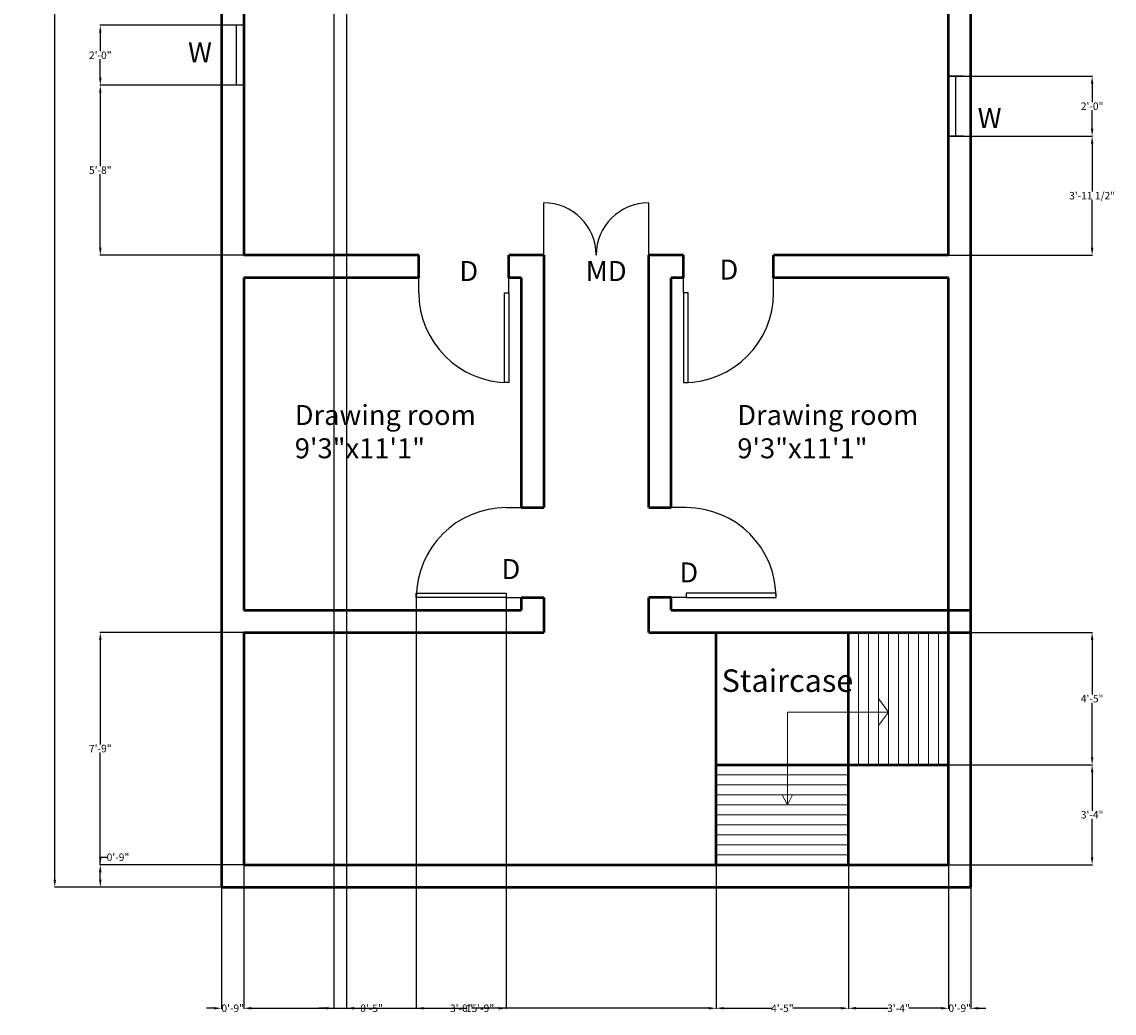
# Model space of a CAD drawing. Units: inches. Extents: x -250 to 2650, y 180 to 1183.
# Tile 2 of 10: x 296 to 733, y 180 to 577. Entities that reach past the tile are written whole.
import ezdxf

# ---------------------------------------------------------------- set-up
doc = ezdxf.new("R2010")
doc.units = ezdxf.units.IN
doc.header["$MEASUREMENT"] = 0
for name, color, linetype, lineweight in [('A-ANNO-DIMS', 2, 'Continuous', 18), ('A-ANNO-TEXT', 7, 'Continuous', 18), ('A-AREA-IDEN', 3, 'Continuous', 18), ('A-DOOR', 4, 'Continuous', 25), ('A-FLOR-STRS', 8, 'Continuous', 18), ('A-GLAZ', 3, 'Continuous', 25), ('A-WALL', 7, 'Continuous', 50)]:
    doc.layers.add(name, color=color, linetype=linetype, lineweight=lineweight)
doc.styles.get("Standard").update_dxf_attribs({"font": 'arial.ttf'})
doc.dimstyles.get("Standard").update_dxf_attribs({"dimtxt": 3, "dimasz": 3, "dimexe": 0.18, "dimexo": 0.0625, "dimgap": 0.09, "dimtad": 0, "dimtih": 1, "dimtoh": 1, "dimdec": 0, "dimzin": 0, "dimdsep": 46, "dimlunit": 3, "dimtxsty": 'Standard', "dimcen": 0.09, "dimadec": 0, "dimazin": 0, "dimtfac": 1, "dimtdec": 0, "dimtofl": 0, "dimtmove": 0, "dimatfit": 3, "dimfxl": 1, "dimtolj": 1, "dimtzin": 0, "dimarcsym": 0})

# ---------------------------------------------------------------- blocks, each defined once
blk = doc.blocks.new('*D16')
at = {"layer": 'A-ANNO-DIMS', "color": 0, "lineweight": -2, "transparency": 16777216}
for p, q in [((376.02, 1070.02), (309.2, 1070.02)), ((309.38, 1067.02), (309.38, 657.77)), ((309.38, 233.02), (309.38, 642.28)), ((376.02, 230.02), (309.2, 230.02))]:
    blk.add_line(p, q, dxfattribs=at)
at = {"layer": 'A-ANNO-DIMS', "color": 0, "transparency": 16777216}
for points in [[(308.88, 1067.02), (309.88, 1067.02), (309.38, 1070.02)], [(308.88, 233.02), (309.88, 233.02), (309.38, 230.02)]]:
    blk.add_solid(points, dxfattribs=at)
at = {"layer": 'Defpoints', "color": 0, "transparency": 16777216}
for p in [(376.08, 1070.02), (309.38, 230.02), (376.08, 230.02)]:
    blk.add_point(p, dxfattribs=at)
at = {"layer": 'A-ANNO-DIMS', "color": 0, "transparency": 16777216, "insert": (309.38, 650.02), "char_height": 3, "attachment_point": 5}
blk.add_mtext("\\A1;{\\H5x;70'}", dxfattribs=at)
blk = doc.blocks.new('*U30')
for p, q in [((-36, 0), (-36, -6)), ((0, 0), (0, -6))]:
    blk.add_line(p, q)
blk.add_lwpolyline([(0, 0), (0, 36), (-1.75, 36), (-1.75, 0)], close=True)
blk.add_arc((0, 0), 36, 90, 180)
blk = doc.blocks.new('*U31')
for p, q in [((-36, 0), (-36, 6)), ((0, 0), (0, 6))]:
    blk.add_line(p, q)
blk.add_lwpolyline([(0, 0), (0, -36), (-1.75, -36), (-1.75, 0)], close=True)
blk.add_arc((0, 0), 36, 180, 270)
blk = doc.blocks.new('*U32')
for p, q in [((0, 0), (0, -6)), ((36, 0), (36, -6))]:
    blk.add_line(p, q)
blk.add_lwpolyline([(0, 0), (0, 36), (1.75, 36), (1.75, 0)], close=True)
blk.add_arc((0, 0), 36, 0, 90)
blk = doc.blocks.new('*U33')
for p, q in [((-36, 0), (-36, -6)), ((0, 0), (0, -6))]:
    blk.add_line(p, q)
blk.add_lwpolyline([(0, 0), (0, 36), (-1.75, 36), (-1.75, 0)], close=True)
blk.add_arc((0, 0), 36, 90, 180)
blk = doc.blocks.new('*U23')
for p, q in [((-24, 6), (-24, 0)), ((0, 6), (0, 0)), ((0, 3), (-24, 3))]:
    blk.add_line(p, q)
blk = doc.blocks.new('*U24')
for p, q in [((-24, 6), (-24, 0)), ((0, 6), (0, 0)), ((0, 3), (-24, 3))]:
    blk.add_line(p, q)
blk = doc.blocks.new('DOOR-DOUBLE-MAIN')
for p, q in [((505.08, 483.11), (505.08, 504.11)), ((505.08, 483.11), (505.08, 504.11)), ((547.08, 483.11), (547.08, 504.11))]:
    blk.add_line(p, q)
for centre, start, end in [((505.08, 483.11), 0, 90), ((505.08, 483.11), 0, 90), ((547.08, 483.11), 90, 180)]:
    blk.add_arc(centre, 21, start, end)
blk = doc.blocks.new('*D72')
at = {"layer": 'A-ANNO-DIMS', "color": 0, "lineweight": -2, "transparency": 16777216}
for p, q in [((667.083902, 238.962048), (667.083902, 181.344548)), ((676.083902, 229.962048), (676.083902, 181.344548)), ((664.083902, 181.524548), (661.083902, 181.524548)), ((679.083902, 181.524548), (682.083902, 181.524548))]:
    blk.add_line(p, q, dxfattribs=at)
at = {"layer": 'A-ANNO-DIMS', "color": 0, "transparency": 16777216}
for points in [[(664.083902, 182.024548), (664.083902, 181.024548), (667.083902, 181.524548)], [(679.083902, 182.024548), (679.083902, 181.024548), (676.083902, 181.524548)]]:
    blk.add_solid(points, dxfattribs=at)
at = {"layer": 'Defpoints', "color": 0, "transparency": 16777216}
for p in [(667.083902, 239.024548), (676.083902, 230.024548), (676.083902, 181.524548)]:
    blk.add_point(p, dxfattribs=at)
at = {"layer": 'A-ANNO-DIMS', "color": 0, "transparency": 16777216, "insert": (671.583902, 181.524548), "char_height": 3, "attachment_point": 5}
blk.add_mtext('\\A1;0\'-9"', dxfattribs=at)
blk = doc.blocks.new('*D73')
at = {"layer": 'A-ANNO-DIMS', "color": 0, "lineweight": -2, "transparency": 16777216}
for p, q in [((385.083902, 238.962048), (385.083902, 181.344548)), ((376.083902, 229.962048), (376.083902, 181.344548)), ((373.083902, 181.524548), (370.083902, 181.524548)), ((388.083902, 181.524548), (391.083902, 181.524548))]:
    blk.add_line(p, q, dxfattribs=at)
at = {"layer": 'A-ANNO-DIMS', "color": 0, "transparency": 16777216}
for points in [[(373.083902, 182.024548), (373.083902, 181.024548), (376.083902, 181.524548)], [(388.083902, 182.024548), (388.083902, 181.024548), (385.083902, 181.524548)]]:
    blk.add_solid(points, dxfattribs=at)
at = {"layer": 'Defpoints', "color": 0, "transparency": 16777216}
for p in [(385.083902, 239.024548), (376.083902, 230.024548), (385.083902, 181.524548)]:
    blk.add_point(p, dxfattribs=at)
at = {"layer": 'A-ANNO-DIMS', "color": 0, "transparency": 16777216, "insert": (380.583902, 181.524548), "char_height": 3, "attachment_point": 5}
blk.add_mtext('\\A1;0\'-9"', dxfattribs=at)
blk = doc.blocks.new('*D74')
at = {"layer": 'A-ANNO-DIMS', "color": 0, "lineweight": -2, "transparency": 16777216}
for p, q in [((385.08, 238.96), (385.08, 181.34)), ((574.08, 238.96), (574.08, 181.34)), ((388.08, 181.52), (474.48, 181.52)), ((571.08, 181.52), (484.69, 181.52))]:
    blk.add_line(p, q, dxfattribs=at)
at = {"layer": 'A-ANNO-DIMS', "color": 0, "transparency": 16777216}
for points in [[(388.08, 182.02), (388.08, 181.02), (385.08, 181.52)], [(571.08, 182.02), (571.08, 181.02), (574.08, 181.52)]]:
    blk.add_solid(points, dxfattribs=at)
at = {"layer": 'Defpoints', "color": 0, "transparency": 16777216}
for p in [(385.08, 239.02), (574.08, 239.02), (574.08, 181.52)]:
    blk.add_point(p, dxfattribs=at)
at = {"layer": 'A-ANNO-DIMS', "color": 0, "transparency": 16777216, "insert": (479.58, 181.52), "char_height": 3, "attachment_point": 5}
blk.add_mtext('\\A1;15\'-9"', dxfattribs=at)
blk = doc.blocks.new('*D75')
at = {"layer": 'A-ANNO-DIMS', "color": 0, "lineweight": -2, "transparency": 16777216}
for p, q in [((574.08, 238.96), (574.08, 181.34)), ((627.08, 238.96), (627.08, 181.34)), ((577.08, 181.52), (596.45, 181.52)), ((624.08, 181.52), (604.72, 181.52))]:
    blk.add_line(p, q, dxfattribs=at)
at = {"layer": 'A-ANNO-DIMS', "color": 0, "transparency": 16777216}
for points in [[(577.08, 182.02), (577.08, 181.02), (574.08, 181.52)], [(624.08, 182.02), (624.08, 181.02), (627.08, 181.52)]]:
    blk.add_solid(points, dxfattribs=at)
at = {"layer": 'Defpoints', "color": 0, "transparency": 16777216}
for p in [(574.08, 239.02), (627.08, 239.02), (627.08, 181.52)]:
    blk.add_point(p, dxfattribs=at)
at = {"layer": 'A-ANNO-DIMS', "color": 0, "transparency": 16777216, "insert": (600.58, 181.52), "char_height": 3, "attachment_point": 5}
blk.add_mtext('\\A1;4\'-5"', dxfattribs=at)
blk = doc.blocks.new('*D76')
at = {"layer": 'A-ANNO-DIMS', "color": 0, "lineweight": -2, "transparency": 16777216}
for p, q in [((627.08, 238.96), (627.08, 181.34)), ((667.08, 238.96), (667.08, 181.34)), ((630.08, 181.52), (643.01, 181.52)), ((664.08, 181.52), (651.16, 181.52))]:
    blk.add_line(p, q, dxfattribs=at)
at = {"layer": 'A-ANNO-DIMS', "color": 0, "transparency": 16777216}
for points in [[(630.08, 182.02), (630.08, 181.02), (627.08, 181.52)], [(664.08, 182.02), (664.08, 181.02), (667.08, 181.52)]]:
    blk.add_solid(points, dxfattribs=at)
at = {"layer": 'Defpoints', "color": 0, "transparency": 16777216}
for p in [(627.08, 239.02), (667.08, 239.02), (667.08, 181.52)]:
    blk.add_point(p, dxfattribs=at)
at = {"layer": 'A-ANNO-DIMS', "color": 0, "transparency": 16777216, "insert": (647.08, 181.52), "char_height": 3, "attachment_point": 5}
blk.add_mtext('\\A1;3\'-4"', dxfattribs=at)
blk = doc.blocks.new('*D77')
at = {"layer": 'A-ANNO-DIMS', "color": 0, "lineweight": -2, "transparency": 16777216}
for p, q in [((667.15, 279.02), (724.76, 279.02)), ((724.58, 276.02), (724.58, 260.65)), ((724.58, 242.02), (724.58, 257.4)), ((667.15, 239.02), (724.76, 239.02))]:
    blk.add_line(p, q, dxfattribs=at)
at = {"layer": 'A-ANNO-DIMS', "color": 0, "transparency": 16777216}
for points in [[(724.08, 276.02), (725.08, 276.02), (724.58, 279.02)], [(724.08, 242.02), (725.08, 242.02), (724.58, 239.02)]]:
    blk.add_solid(points, dxfattribs=at)
at = {"layer": 'Defpoints', "color": 0, "transparency": 16777216}
for p in [(667.08, 279.02), (724.58, 279.02), (667.08, 239.02)]:
    blk.add_point(p, dxfattribs=at)
at = {"layer": 'A-ANNO-DIMS', "color": 0, "transparency": 16777216, "insert": (724.58, 259.02), "char_height": 3, "attachment_point": 5}
blk.add_mtext('\\A1;3\'-4"', dxfattribs=at)
blk = doc.blocks.new('*D78')
at = {"layer": 'A-ANNO-DIMS', "color": 0, "lineweight": -2, "transparency": 16777216}
for p, q in [((663.15, 332.02), (724.76, 332.02)), ((724.58, 329.02), (724.58, 307.14)), ((724.58, 282.02), (724.58, 303.91)), ((667.15, 279.02), (724.76, 279.02))]:
    blk.add_line(p, q, dxfattribs=at)
at = {"layer": 'A-ANNO-DIMS', "color": 0, "transparency": 16777216}
for points in [[(724.08, 329.02), (725.08, 329.02), (724.58, 332.02)], [(724.08, 282.02), (725.08, 282.02), (724.58, 279.02)]]:
    blk.add_solid(points, dxfattribs=at)
at = {"layer": 'Defpoints', "color": 0, "transparency": 16777216}
for p in [(663.08, 332.02), (724.58, 332.02), (667.08, 279.02)]:
    blk.add_point(p, dxfattribs=at)
at = {"layer": 'A-ANNO-DIMS', "color": 0, "transparency": 16777216, "insert": (724.58, 305.52), "char_height": 3, "attachment_point": 5}
blk.add_mtext('\\A1;4\'-5"', dxfattribs=at)
blk = doc.blocks.new('*D79')
at = {"layer": 'A-ANNO-DIMS', "color": 0, "lineweight": -2, "transparency": 16777216}
for p, q in [((327.58, 239.02), (327.58, 242.02)), ((327.58, 242.02), (330.58, 242.02)), ((385.02, 239.02), (327.4, 239.02)), ((327.58, 233.02), (327.58, 236.02)), ((376.02, 230.02), (327.4, 230.02))]:
    blk.add_line(p, q, dxfattribs=at)
at = {"layer": 'A-ANNO-DIMS', "color": 0, "transparency": 16777216}
for points in [[(327.08, 236.02), (328.08, 236.02), (327.58, 239.02)], [(327.08, 233.02), (328.08, 233.02), (327.58, 230.02)]]:
    blk.add_solid(points, dxfattribs=at)
at = {"layer": 'Defpoints', "color": 0, "transparency": 16777216}
for p in [(327.58, 239.02), (385.08, 239.02), (376.08, 230.02)]:
    blk.add_point(p, dxfattribs=at)
at = {"layer": 'A-ANNO-DIMS', "color": 0, "transparency": 16777216, "insert": (334.66, 242.02), "char_height": 3, "attachment_point": 5}
blk.add_mtext('\\A1;0\'-9"', dxfattribs=at)
blk = doc.blocks.new('*D80')
at = {"layer": 'A-ANNO-DIMS', "color": 0, "lineweight": -2, "transparency": 16777216}
for p, q in [((385.02, 332.02), (327.4, 332.02)), ((327.58, 329.02), (327.58, 287.15)), ((327.58, 242.02), (327.58, 283.9)), ((385.02, 239.02), (327.4, 239.02))]:
    blk.add_line(p, q, dxfattribs=at)
at = {"layer": 'A-ANNO-DIMS', "color": 0, "transparency": 16777216}
for points in [[(327.08, 329.02), (328.08, 329.02), (327.58, 332.02)], [(327.08, 242.02), (328.08, 242.02), (327.58, 239.02)]]:
    blk.add_solid(points, dxfattribs=at)
at = {"layer": 'Defpoints', "color": 0, "transparency": 16777216}
for p in [(327.58, 332.02), (385.08, 332.02), (385.08, 239.02)]:
    blk.add_point(p, dxfattribs=at)
at = {"layer": 'A-ANNO-DIMS', "color": 0, "transparency": 16777216, "insert": (327.58, 285.52), "char_height": 3, "attachment_point": 5}
blk.add_mtext('\\A1;7\'-9"', dxfattribs=at)
blk = doc.blocks.new('*D82')
at = {"layer": 'A-ANNO-DIMS', "color": 0, "lineweight": -2, "transparency": 16777216}
for p, q in [((421.09, 643.56), (421.09, 181.34)), ((426.08, 639.05), (426.08, 181.34)), ((418.09, 181.52), (415.09, 181.52)), ((429.08, 181.52), (432.08, 181.52))]:
    blk.add_line(p, q, dxfattribs=at)
at = {"layer": 'A-ANNO-DIMS', "color": 0, "transparency": 16777216}
for points in [[(418.09, 182.02), (418.09, 181.02), (421.09, 181.52)], [(429.08, 182.02), (429.08, 181.02), (426.08, 181.52)]]:
    blk.add_solid(points, dxfattribs=at)
at = {"layer": 'Defpoints', "color": 0, "transparency": 16777216}
for p in [(421.09, 643.62), (426.08, 639.11), (426.08, 181.52)]:
    blk.add_point(p, dxfattribs=at)
at = {"layer": 'A-ANNO-DIMS', "color": 0, "transparency": 16777216, "insert": (436.16, 181.52), "char_height": 3, "attachment_point": 5}
blk.add_mtext('\\A1;0\'-5"', dxfattribs=at)
blk = doc.blocks.new('*D85')
at = {"layer": 'A-ANNO-DIMS', "color": 0, "lineweight": -2, "transparency": 16777216}
for p, q in [((667.15, 530.79), (724.76, 530.79)), ((724.58, 527.79), (724.58, 508.59)), ((724.58, 486.11), (724.58, 505.31)), ((667.15, 483.11), (724.76, 483.11))]:
    blk.add_line(p, q, dxfattribs=at)
at = {"layer": 'A-ANNO-DIMS', "color": 0, "transparency": 16777216}
for points in [[(724.08, 527.79), (725.08, 527.79), (724.58, 530.79)], [(724.08, 486.11), (725.08, 486.11), (724.58, 483.11)]]:
    blk.add_solid(points, dxfattribs=at)
at = {"layer": 'Defpoints', "color": 0, "transparency": 16777216}
for p in [(667.08, 530.79), (724.58, 530.79), (667.08, 483.11)]:
    blk.add_point(p, dxfattribs=at)
at = {"layer": 'A-ANNO-DIMS', "color": 0, "transparency": 16777216, "insert": (724.58, 506.95), "char_height": 3, "attachment_point": 5}
blk.add_mtext('\\A1;3\'-11 1/2"', dxfattribs=at)
blk = doc.blocks.new('*D86')
at = {"layer": 'A-ANNO-DIMS', "color": 0, "lineweight": -2, "transparency": 16777216}
for p, q in [((667.15, 554.79), (724.76, 554.79)), ((724.58, 551.79), (724.58, 544.41)), ((724.58, 533.79), (724.58, 541.16)), ((667.15, 530.79), (724.76, 530.79))]:
    blk.add_line(p, q, dxfattribs=at)
at = {"layer": 'A-ANNO-DIMS', "color": 0, "transparency": 16777216}
for points in [[(724.08, 551.79), (725.08, 551.79), (724.58, 554.79)], [(724.08, 533.79), (725.08, 533.79), (724.58, 530.79)]]:
    blk.add_solid(points, dxfattribs=at)
at = {"layer": 'Defpoints', "color": 0, "transparency": 16777216}
for p in [(667.08, 554.79), (724.58, 554.79), (667.08, 530.79)]:
    blk.add_point(p, dxfattribs=at)
at = {"layer": 'A-ANNO-DIMS', "color": 0, "transparency": 16777216, "insert": (724.58, 542.79), "char_height": 3, "attachment_point": 5}
blk.add_mtext('\\A1;2\'-0"', dxfattribs=at)
blk = doc.blocks.new('*D87')
at = {"layer": 'A-ANNO-DIMS', "color": 0, "lineweight": -2, "transparency": 16777216}
for p, q in [((385.02, 551.2), (327.4, 551.2)), ((327.58, 548.2), (327.58, 518.78)), ((327.58, 486.11), (327.58, 515.53)), ((385.02, 483.11), (327.4, 483.11))]:
    blk.add_line(p, q, dxfattribs=at)
at = {"layer": 'A-ANNO-DIMS', "color": 0, "transparency": 16777216}
for points in [[(327.08, 548.2), (328.08, 548.2), (327.58, 551.2)], [(327.08, 486.11), (328.08, 486.11), (327.58, 483.11)]]:
    blk.add_solid(points, dxfattribs=at)
at = {"layer": 'Defpoints', "color": 0, "transparency": 16777216}
for p in [(327.58, 551.2), (385.08, 551.2), (385.08, 483.11)]:
    blk.add_point(p, dxfattribs=at)
at = {"layer": 'A-ANNO-DIMS', "color": 0, "transparency": 16777216, "insert": (327.58, 517.16), "char_height": 3, "attachment_point": 5}
blk.add_mtext('\\A1;5\'-8"', dxfattribs=at)
blk = doc.blocks.new('*D88')
at = {"layer": 'A-ANNO-DIMS', "color": 0, "lineweight": -2, "transparency": 16777216}
for p, q in [((385.02, 575.2), (327.4, 575.2)), ((327.58, 572.2), (327.58, 564.82)), ((327.58, 554.2), (327.58, 561.58)), ((385.02, 551.2), (327.4, 551.2))]:
    blk.add_line(p, q, dxfattribs=at)
at = {"layer": 'A-ANNO-DIMS', "color": 0, "transparency": 16777216}
for points in [[(327.08, 572.2), (328.08, 572.2), (327.58, 575.2)], [(327.08, 554.2), (328.08, 554.2), (327.58, 551.2)]]:
    blk.add_solid(points, dxfattribs=at)
at = {"layer": 'Defpoints', "color": 0, "transparency": 16777216}
for p in [(327.58, 575.2), (385.08, 575.2), (385.08, 551.2)]:
    blk.add_point(p, dxfattribs=at)
at = {"layer": 'A-ANNO-DIMS', "color": 0, "transparency": 16777216, "insert": (327.58, 563.2), "char_height": 3, "attachment_point": 5}
blk.add_mtext('\\A1;2\'-0"', dxfattribs=at)
blk = doc.blocks.new('*D89')
at = {"layer": 'A-ANNO-DIMS', "color": 0, "lineweight": -2, "transparency": 16777216}
for p, q in [((454.08, 345.96), (454.08, 181.34)), ((490.08, 345.96), (490.08, 181.34)), ((457.08, 181.52), (468.01, 181.52)), ((487.08, 181.52), (476.16, 181.52))]:
    blk.add_line(p, q, dxfattribs=at)
at = {"layer": 'A-ANNO-DIMS', "color": 0, "transparency": 16777216}
for points in [[(457.08, 182.02), (457.08, 181.02), (454.08, 181.52)], [(487.08, 182.02), (487.08, 181.02), (490.08, 181.52)]]:
    blk.add_solid(points, dxfattribs=at)
at = {"layer": 'Defpoints', "color": 0, "transparency": 16777216}
for p in [(454.08, 346.02), (490.08, 346.02), (490.08, 181.52)]:
    blk.add_point(p, dxfattribs=at)
at = {"layer": 'A-ANNO-DIMS', "color": 0, "transparency": 16777216, "insert": (472.08, 181.52), "char_height": 3, "attachment_point": 5}
blk.add_mtext('\\A1;3\'-0"', dxfattribs=at)

msp = doc.modelspace()

# ---------------------------------------------------------------- linework, layer by layer
at = {"layer": 'A-FLOR-STRS'}
for p, q in [((631.08, 279.02), (631.08, 332.02)), ((635.08, 279.02), (635.08, 332.02)), ((639.08, 279.02), (639.08, 332.02)), ((643.08, 279.02), (643.08, 332.02)), ((647.08, 279.02), (647.08, 332.02)), ((651.08, 279.02), (651.08, 332.02)), ((655.08, 279.02), (655.08, 332.02)), ((659.08, 279.02), (659.08, 332.02)), ((663.08, 279.02), (663.08, 332.02)), ((643.08, 300.14), (639.08, 305.52)), ((602.6, 300.14), (602.6, 263.02)), ((602.6, 300.14), (643.08, 300.14)), ((643.08, 300.14), (639.08, 294.75)), ((574.08, 275.02), (627.08, 275.02)), ((574.08, 271.02), (627.08, 271.02)), ((574.08, 267.02), (627.08, 267.02)), ((602.6, 263.02), (600.58, 267.02)), ((602.6, 263.02), (604.61, 267.02)), ((574.08, 263.02), (627.08, 263.02)), ((574.08, 259.02), (627.08, 259.02)), ((574.08, 255.02), (627.08, 255.02)), ((574.08, 251.02), (627.08, 251.02)), ((574.08, 247.02), (627.08, 247.02)), ((574.08, 243.02), (627.08, 243.02))]:
    msp.add_line(p, q, dxfattribs=at)
at = {"layer": 'A-WALL'}
for p, q in [((376.08, 1070.02), (376.08, 230.02)), ((676.08, 230.02), (676.08, 1070.02)), ((385.08, 639.11), (385.08, 483.11)), ((667.08, 483.11), (667.08, 639.11)), ((455.08, 483.11), (385.08, 483.11)), ((455.08, 474.11), (455.08, 483.11)), ((491.08, 474.11), (491.08, 483.11)), ((505.08, 483.11), (491.08, 483.11)), ((505.08, 483.11), (505.08, 382.02)), ((547.08, 382.02), (547.08, 483.11)), ((561.08, 483.11), (547.08, 483.11)), ((561.08, 474.11), (561.08, 483.11)), ((667.08, 483.11), (597.08, 483.11)), ((597.08, 474.11), (597.08, 483.11)), ((385.08, 474.11), (385.08, 341.02)), ((455.08, 474.11), (385.08, 474.11)), ((496.08, 474.11), (491.08, 474.11)), ((496.08, 474.11), (496.08, 382.02)), ((556.08, 382.02), (556.08, 474.11)), ((561.08, 474.11), (556.08, 474.11)), ((667.08, 474.11), (597.08, 474.11)), ((667.08, 239.02), (667.08, 474.11)), ((496.08, 382.02), (505.08, 382.02)), ((547.08, 382.02), (556.08, 382.02)), ((496.08, 346.02), (505.08, 346.02)), ((496.08, 346.02), (496.08, 341.02)), ((505.08, 346.02), (505.08, 332.02)), ((547.08, 332.02), (547.08, 346.02)), ((556.08, 346.02), (547.08, 346.02)), ((556.08, 341.02), (556.08, 346.02)), ((385.08, 341.02), (496.08, 341.02)), ((556.08, 341.02), (676.08, 341.02)), ((385.08, 332.02), (385.08, 239.02)), ((385.08, 332.02), (505.08, 332.02)), ((547.08, 332.02), (676.08, 332.02)), ((574.08, 239.02), (574.08, 332.02)), ((627.08, 239.02), (627.08, 332.02)), ((574.08, 279.02), (667.08, 279.02)), ((385.08, 239.02), (409.83, 239.02)), ((385.08, 239.02), (667.08, 239.02)), ((376.08, 230.02), (409.08, 230.02)), ((376.08, 230.02), (676.08, 230.02))]:
    msp.add_line(p, q, dxfattribs=at)

# ---------------------------------------------------------------- block references
at = {"layer": 'A-DOOR'}
msp.add_blockref('DOOR-DOUBLE-MAIN', (0, 0), dxfattribs=at)
for name, p, rotation in [('*U32', (491.08, 468.11), 180), ('*U33', (561.08, 468.11), 180), ('*U31', (490.08, 346.02), 270), ('*U30', (562.08, 346.02), 270)]:
    msp.add_blockref(name, p, dxfattribs=dict(at, rotation=rotation))
at = {"layer": 'A-GLAZ', "rotation": 270}
for name, p in [('*U23', (379.08, 551.2)), ('*U24', (667.08, 530.79))]:
    msp.add_blockref(name, p, dxfattribs=at)

# ---------------------------------------------------------------- texts
at = {"layer": 'A-ANNO-TEXT', "char_height": 8, "attachment_point": 1}
for s, insert in [('W', (362.69, 568.43)), ('W', (678.76, 542.11)), ('D', (575.44, 481.35)), ('D', (471.32, 480.78)), ('MD', (521.89, 480.78)), ('D', (488.19, 361.42)), ('D', (559.39, 360.07))]:
    msp.add_mtext_dynamic_manual_height_columns(s, width=10.3916, gutter_width=1, heights=[0], dxfattribs=dict(at, insert=insert))
at = {"layer": 'A-AREA-IDEN', "attachment_point": 1}
for s, width, insert, char_height in [('Drawing room 9\'3"x11\'1"', 88.0689, (405.43, 423.12), 8), ('Drawing room 9\'3"x11\'1"', 88.0689, (582.56, 423.12), 8), ('Staircase  ', 87.4783, (576.26, 317.24), 9)]:
    msp.add_mtext_dynamic_manual_height_columns(s, width=width, gutter_width=1, heights=[0], dxfattribs=dict(at, insert=insert, char_height=char_height))

# ---------------------------------------------------------------- dimensions: what is measured, and where the dimension line sits
at = {"layer": 'A-ANNO-DIMS'}
dim = msp.add_linear_dim(base=(309.38, 230.02), p1=(376.08, 1070.02), p2=(376.08, 230.02), angle=90, text='{\\H5x;<>}', dimstyle='Standard', override={"dimclrd": 0, "dimclre": 0, "dimclrt": 0}, dxfattribs=at)
dim.commit()
dim.dimension.update_dxf_attribs({"geometry": '*D16', "text_midpoint": (309.38, 650.02)})
for base, p1, p2, picture, middle in [((426.08, 181.52), (421.09, 643.62), (426.08, 639.11), '*D82', (436.16, 181.52)), ((490.08, 181.52), (454.08, 346.02), (490.08, 346.02), '*D89', (472.08, 181.52)), ((385.08, 181.52), (376.08, 230.02), (385.08, 239.02), '*D73', (380.58, 181.52)), ((574.08, 181.52), (385.08, 239.02), (574.08, 239.02), '*D74', (479.58, 181.52)), ((627.08, 181.52), (574.08, 239.02), (627.08, 239.02), '*D75', (600.58, 181.52)), ((667.08, 181.52), (627.08, 239.02), (667.08, 239.02), '*D76', (647.08, 181.52)), ((676.08, 181.52), (667.08, 239.02), (676.08, 230.02), '*D72', (671.58, 181.52))]:
    dim = msp.add_linear_dim(base=base, p1=p1, p2=p2, dimstyle='Standard', override={"dimdec": 1, "dimlfac": 1, "dimrnd": 0, "dimzin": 1, "dimdsep": 46, "dimlunit": 4, "dimfrac": 2}, dxfattribs=at)
    dim.commit()
    dim.dimension.update_dxf_attribs({"geometry": picture, "text_midpoint": middle})
for base, p1, p2, picture, middle in [((327.58, 575.2), (385.08, 551.2), (385.08, 575.2), '*D88', (327.58, 563.2)), ((327.58, 551.2), (385.08, 483.11), (385.08, 551.2), '*D87', (327.58, 517.16)), ((724.58, 554.79), (667.08, 530.79), (667.08, 554.79), '*D86', (724.58, 542.79)), ((724.58, 530.79), (667.08, 483.11), (667.08, 530.79), '*D85', (724.58, 506.95)), ((327.58, 332.02), (385.08, 239.02), (385.08, 332.02), '*D80', (327.58, 285.52)), ((724.58, 332.02), (667.08, 279.02), (663.08, 332.02), '*D78', (724.58, 305.52)), ((724.58, 279.02), (667.08, 239.02), (667.08, 279.02), '*D77', (724.58, 259.02)), ((327.58, 239.02), (376.08, 230.02), (385.08, 239.02), '*D79', (334.66, 242.02))]:
    dim = msp.add_linear_dim(base=base, p1=p1, p2=p2, angle=90, dimstyle='Standard', override={"dimdec": 1, "dimlfac": 1, "dimrnd": 0, "dimzin": 1, "dimdsep": 46, "dimlunit": 4, "dimfrac": 2}, dxfattribs=at)
    dim.commit()
    dim.dimension.update_dxf_attribs({"geometry": picture, "text_midpoint": middle})

doc.saveas('drawing.dxf')
